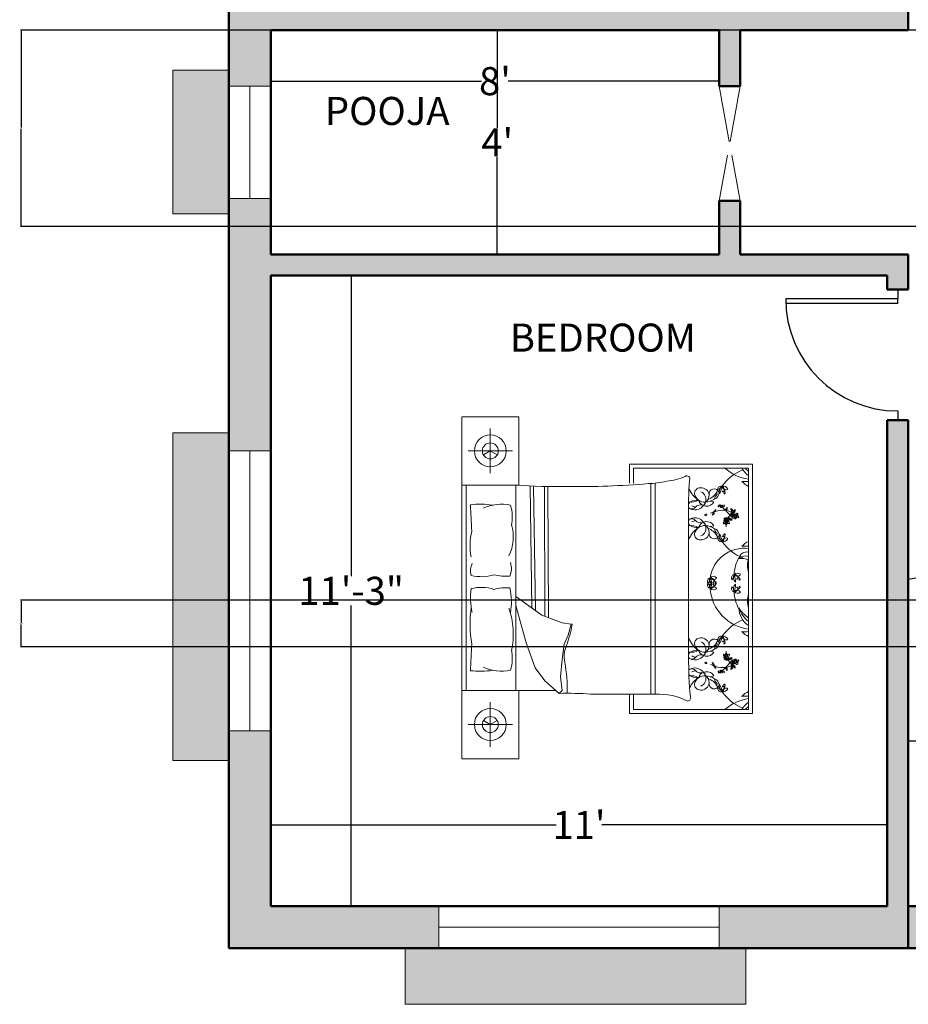
# Model space of a CAD drawing. Units: inches. Extents: x -28 to 544, y -640 to 52.
# Tile 1 of 11: x -28 to 162, y -600 to -389. Entities that reach past the tile are written whole.
import ezdxf

# ---------------------------------------------------------------- set-up
doc = ezdxf.new("R2010")
doc.units = ezdxf.units.IN
doc.header["$MEASUREMENT"] = 0
doc.linetypes.add('ACAD_ISO02W100', pattern=[15, 12, -3])
for name, color, linetype, lineweight in [('A-ANNO-DIMS', 2, 'Continuous', 18), ('A-AREA-IDEN', 7, 'Continuous', 25), ('A-DOOR', 3, 'Continuous', 25), ('A-FURN', 8, 'Continuous', 18), ('A-GLAZ', 4, 'Continuous', 20), ('A-ROOF', 8, 'Continuous', 18), ('A-ROOF-PATT', 252, 'Continuous', 13), ('A-WALL', 7, 'Continuous', 50), ('A-WALL-OVHD', 8, 'ACAD_ISO02W100', 18), ('A-WALL-PATT', 5, 'Continuous', 13)]:
    doc.layers.add(name, color=color, linetype=linetype, lineweight=lineweight)
doc.styles.get("Standard").update_dxf_attribs({"font": 'arial.ttf'})
doc.dimstyles.get("Standard").update_dxf_attribs({"dimtxt": 0.18, "dimasz": 0.18, "dimexe": 0.18, "dimexo": 0.0625, "dimgap": 0.09, "dimtad": 0, "dimtih": 1, "dimtoh": 1, "dimdec": 0, "dimzin": 0, "dimdsep": 46, "dimlunit": 3, "dimtxsty": 'Standard', "dimcen": 0.09, "dimadec": 0, "dimazin": 0, "dimtfac": 1, "dimtdec": 0, "dimtofl": 0, "dimtmove": 0, "dimatfit": 3, "dimfxl": 1, "dimtolj": 1, "dimtzin": 0, "dimarcsym": 0})

# ---------------------------------------------------------------- blocks, each defined once
blk = doc.blocks.new('*D21')
at = {"layer": 'A-ANNO-DIMS', "color": 0, "lineweight": -2, "transparency": 16777216}
for p, q in [((42.28, -443.74), (43.33, -443.74)), ((43.15, -443.92), (43.15, -508.09)), ((43.15, -578.56), (43.15, -514.4)), ((42.28, -578.74), (43.33, -578.74))]:
    blk.add_line(p, q, dxfattribs=at)
at = {"layer": 'A-ANNO-DIMS', "color": 0, "transparency": 16777216}
for points in [[(43.12, -443.92), (43.18, -443.92), (43.15, -443.74)], [(43.12, -578.56), (43.18, -578.56), (43.15, -578.74)]]:
    blk.add_solid(points, dxfattribs=at)
at = {"layer": 'Defpoints', "color": 0, "transparency": 16777216}
for p in [(42.22, -443.74), (42.22, -578.74), (43.15, -578.74)]:
    blk.add_point(p, dxfattribs=at)
at = {"layer": 'A-ANNO-DIMS', "color": 0, "transparency": 16777216, "insert": (43.15, -511.24), "char_height": 6, "attachment_point": 5}
blk.add_mtext('\\A1;11\'-3"', dxfattribs=at)
blk = doc.blocks.new('*D22')
at = {"layer": 'A-ANNO-DIMS', "color": 0, "lineweight": -2, "transparency": 16777216}
for p, q in [((25.94, -561.29), (25.94, -561.17)), ((26.12, -561.35), (87.05, -561.35)), ((157.76, -561.35), (96.84, -561.35)), ((157.94, -561.29), (157.94, -561.17))]:
    blk.add_line(p, q, dxfattribs=at)
at = {"layer": 'A-ANNO-DIMS', "color": 0, "transparency": 16777216}
for points in [[(26.12, -561.32), (26.12, -561.38), (25.94, -561.35)], [(157.76, -561.32), (157.76, -561.38), (157.94, -561.35)]]:
    blk.add_solid(points, dxfattribs=at)
at = {"layer": 'Defpoints', "color": 0, "transparency": 16777216}
for p in [(25.94, -561.35), (157.94, -561.35), (157.94, -561.35)]:
    blk.add_point(p, dxfattribs=at)
at = {"layer": 'A-ANNO-DIMS', "color": 0, "transparency": 16777216, "insert": (91.94, -561.35), "char_height": 6, "attachment_point": 5}
blk.add_mtext("\\A1;11'", dxfattribs=at)
blk = doc.blocks.new('*D29')
at = {"layer": 'A-ANNO-DIMS', "color": 0, "lineweight": -2, "transparency": 16777216}
for p, q in [((75.12, -391.24), (74.25, -391.24)), ((74.43, -391.42), (74.43, -412.15)), ((74.43, -439.06), (74.43, -418.33)), ((75.12, -439.24), (74.25, -439.24))]:
    blk.add_line(p, q, dxfattribs=at)
at = {"layer": 'A-ANNO-DIMS', "color": 0, "transparency": 16777216}
for points in [[(74.4, -391.42), (74.46, -391.42), (74.43, -391.24)], [(74.4, -439.06), (74.46, -439.06), (74.43, -439.24)]]:
    blk.add_solid(points, dxfattribs=at)
at = {"layer": 'Defpoints', "color": 0, "transparency": 16777216}
for p in [(75.19, -391.24), (74.43, -439.24), (75.19, -439.24)]:
    blk.add_point(p, dxfattribs=at)
at = {"layer": 'A-ANNO-DIMS', "color": 0, "transparency": 16777216, "insert": (74.43, -415.24), "char_height": 6, "attachment_point": 5}
blk.add_mtext("\\A1;4'", dxfattribs=at)
blk = doc.blocks.new('*D30')
at = {"layer": 'A-ANNO-DIMS', "color": 0, "lineweight": -2, "transparency": 16777216}
for p, q in [((25.94, -427.18), (25.94, -401.96)), ((26.12, -402.14), (71.09, -402.14)), ((121.76, -402.14), (76.8, -402.14)), ((121.94, -401.16), (121.94, -402.32))]:
    blk.add_line(p, q, dxfattribs=at)
at = {"layer": 'A-ANNO-DIMS', "color": 0, "transparency": 16777216}
for points in [[(26.12, -402.11), (26.12, -402.17), (25.94, -402.14)], [(121.76, -402.11), (121.76, -402.17), (121.94, -402.14)]]:
    blk.add_solid(points, dxfattribs=at)
at = {"layer": 'Defpoints', "color": 0, "transparency": 16777216}
for p in [(121.94, -401.09), (121.94, -402.14), (25.94, -427.24)]:
    blk.add_point(p, dxfattribs=at)
at = {"layer": 'A-ANNO-DIMS', "color": 0, "transparency": 16777216, "insert": (73.94, -402.14), "char_height": 6, "attachment_point": 5}
blk.add_mtext("\\A1;8'", dxfattribs=at)
blk = doc.blocks.new('*D41')
at = {"layer": 'A-ANNO-DIMS', "color": 0, "lineweight": -2, "transparency": 16777216}
for p, q in [((162.44, -543.27), (162.44, -543.15)), ((162.62, -543.33), (238.58, -543.33)), ((334.76, -543.33), (258.81, -543.33)), ((334.94, -543.27), (334.94, -543.15))]:
    blk.add_line(p, q, dxfattribs=at)
at = {"layer": 'A-ANNO-DIMS', "color": 0, "transparency": 16777216}
for points in [[(162.62, -543.3), (162.62, -543.36), (162.44, -543.33)], [(334.76, -543.3), (334.76, -543.36), (334.94, -543.33)]]:
    blk.add_solid(points, dxfattribs=at)
at = {"layer": 'Defpoints', "color": 0, "transparency": 16777216}
for p in [(162.44, -543.33), (334.94, -543.33), (334.94, -543.33)]:
    blk.add_point(p, dxfattribs=at)
at = {"layer": 'A-ANNO-DIMS', "color": 0, "transparency": 16777216, "insert": (248.69, -543.33), "char_height": 6, "attachment_point": 5}
blk.add_mtext('\\A1;14\'-5"', dxfattribs=at)
blk = doc.blocks.new('BED-DOUBLE-HEADBOARD-73')
for p, q in [((0, 0), (0, 73.21)), ((6.1, 61.11), (6.1, 70.67)), ((10.88, 65.89), (1.32, 65.89)), ((35.89, 58.98), (35.89, 63.04)), ((35.89, 63.04), (62.26, 63.04)), ((36.74, 62.19), (36.74, 58.96)), ((61.41, 62.19), (36.74, 62.19)), ((61.41, 10.51), (61.41, 62.19)), ((62.26, 63.04), (62.26, 9.66)), ((0.94, 58.57), (0.94, 14.64)), ((11.57, 14.64), (11.57, 58.57)), ((14.61, 58.37), (14.98, 32.31)), ((15.36, 58.34), (15.74, 31.76)), ((17.67, 58.31), (17.78, 30.51)), ((18.42, 58.31), (18.53, 30.22)), ((40.45, 58.9), (40.45, 13.8)), ((41.37, 58.97), (41.37, 13.8)), ((53.99, 54.97), (53.16, 55.14)), ((48.56, 51.47), (48.56, 21.74)), ((53.99, 49.86), (53.16, 49.7)), ((11.57, 34.76), (17.15, 30.74)), ((13.75, 24.81), (11.57, 32.8)), ((17.15, 30.74), (21.45, 29.11)), ((21.45, 29.11), (23.38, 28.82)), ((23.38, 28.82), (22.79, 26.44)), ((22.79, 26.44), (21.9, 24.52)), ((15.67, 19.47), (13.75, 24.81)), ((21.9, 24.52), (21.45, 21.25)), ((21.45, 21.25), (21.15, 17.55)), ((53.99, 22.84), (53.16, 23)), ((17.75, 16.66), (15.67, 19.47)), ((21.15, 17.55), (21.45, 14.58)), ((53.99, 17.73), (53.16, 17.56)), ((20.86, 13.99), (17.75, 16.66)), ((0, 14.64), (20.09, 14.64)), ((21.45, 14.58), (20.86, 13.99)), ((35.89, 9.66), (35.89, 13.8)), ((36.74, 13.8), (36.74, 10.51)), ((6.1, 12.1), (6.1, 2.54)), ((62.26, 9.66), (35.89, 9.66)), ((36.74, 10.51), (61.41, 10.51)), ((10.88, 7.32), (1.32, 7.32))]:
    blk.add_line(p, q)
for points in [[(0, 58.57), (12.2, 58.57), (12.2, 73.21), (0, 73.21)], [(6.1, 65.89), (4.62, 65.04)], [(6.1, 65.89), (7.58, 65.04)], [(12.2, 14.64), (12.2, 0), (0, 0)], [(6.1, 7.32), (4.62, 8.18)], [(6.1, 7.32), (7.58, 8.18)]]:
    blk.add_lwpolyline(points)
for points in [[(39.88, 58.88, 0.056112), (43.91, 59.41, 0.095341), (47.79, 60.44)], [(1.82, 54.36, -0.074897), (6.61, 54.28, 0.472817)], [(6.87, 39.39, -0.14099), (2, 39.24, -0.235245)], [(6.87, 36.26, 0.14099), (2, 36.41, 0.235245)], [(1.82, 18.85, 0.074897), (6.61, 18.94, -0.472817)], [(27.56, 13.83, 0.001242), (41.45, 13.8, -0.127202), (48.38, 12.33)]]:
    blk.add_lwpolyline(points, format="xyb")
for centre, radius in [((6.1, 65.89), 3.42), ((6.1, 65.89), 1.71), ((56.64, 50.74), 0.186), ((58.61, 51.96), 0.186), ((56.64, 21.96), 0.186), ((58.61, 20.74), 0.186), ((6.1, 7.32), 3.42), ((6.1, 7.32), 1.71)]:
    blk.add_circle(centre, radius)
for centre, radius, start, end in [((63.65, 52.95), 9.56, 111.4092, 145.6135), ((62.7, 69.31), 9.56, 228.1144, 262.255), ((63.98, 64.51), 4.66, 209.8884, 236.5383), ((64.85, 66.19), 5.81, 223.5186, 233.6964), ((48.16, 59.89), 0.667, 336.5219, 123.8264), ((119.76, 53.71), 71.24, 175.2402, 181.8035), ((62.9, 61.9), 3.89, 221.0454, 247.4453), ((60.81, 72.55), 13.23, 266.3481, 272.5919), ((20.52, 189.81), 131.55, 266.1, 270.9282), ((25.3, 229.86), 171.6, 269.1145, 274.8735), ((53.71, 59.98), 5.54, 203.6453, 236.3329), ((51.05, 56.75), 1.24, 88.9462, 185.5144), ((51.23, 56.25), 1.75, 7.1143, 95.0551), ((50.57, 55.56), 1.7, 338.5779, 68.4181), ((51.63, 58.83), 3.46, 288.2955, 328.7386), ((54.05, 56.65), 1.1, 19.1312, 189.736), ((53.72, 56.91), 1.37, 285.6955, 4.031), ((55.24, 56.88), 0.673, 126.7319, 206.0245), ((55.57, 57.58), 0.793, 76.272, 177.0484), ((54.36, 59.2), 1.63, 284.7031, 328.6173), ((56.64, 57.12), 1.51, 125.7657, 194.5347), ((49.23, 59.8), 6.69, 332.8176, 347.4827), ((55.98, 57.31), 1.06, 20.9613, 102.2885), ((56.55, 58.37), 0.798, 181.7131, 301.5367), ((53.94, 56.76), 2.42, 2.0648, 41.1598), ((55.39, 57.66), 0.782, 316.2238, 62.3173), ((55.84, 57.2), 0.0623, 20.2667, 316.2271), ((56.17, 56.85), 0.0577, 52.0591, 168.5166), ((49.1, 57.95), 3.03, 259.249, 301.1782), ((49.37, 54.19), 0.882, 127.675, 162.5814), ((49.89, 55.6), 2.33, 240.8249, 340.7178), ((50.42, 52.56), 2.82, 85.2696, 124.215), ((51.97, 57.13), 2.2, 193.079, 274.7067), ((52.41, 55.88), 1.82, 196.8663, 330.0915), ((51.65, 54.73), 0.454, 254.8529, 12.6959), ((50.42, 52.56), 2.82, 53.6555, 57.2989), ((50.84, 56.55), 2.13, 305.9599, 357.6409), ((51.91, 58.86), 3.93, 273.4924, 303.7117), ((55.54, 55.43), 1.46, 128.4175, 173.8338), ((56.23, 56.84), 0.119, 168.5166, 2.0648), ((-694.9, 14.01), 697.9, 2.85022, 3.31479), ((8.53, 45.04), 9.44, 78.2417, 114.8684), ((0.97, 51.75), 9.81, 348.9631, 14.8961), ((49.37, 54.19), 0.882, 196.6343, 225.5483), ((49.19, 54.56), 1.1, 246.1646, 318.4347), ((50.31, 55.95), 2.1, 240.0851, 262.564), ((51.14, 52.84), 1.5, 74.8529, 138.4347), ((56.02, 47.13), 6.06, 110.1059, 116.9968), ((53.95, 52.6), 0.149, 83.9457, 185.6216), ((53.35, 52.74), 0.614, 328.836, 0.8141), ((53.67, 52.56), 0.351, 306.5232, 32.4668), ((54.09, 52.83), 0.149, 112.5583, 214.2343), ((53.99, 53.1), 0.351, 265.7131, 351.6568), ((53.68, 53.29), 0.614, 297.3659, 329.344), ((53.22, 53.82), 1.18, 313.6929, 321.7899), ((54.52, 53.01), 0.384, 115.5379, 168.6744), ((53.21, 53.57), 1.16, 329.344, 349.7412), ((56.02, 47.13), 6.06, 86.1723, 106.4158), ((52.29, 53.3), 2.06, 352.8698, 1.6736), ((55.02, 54.05), 0.144, 125.0752, 284.7644), ((55.25, 54.1), 0.311, 127.3642, 168.4363), ((55, 54.35), 0.448, 277.4968, 341.2737), ((55.36, 54.14), 0.178, 88.1325, 178.8919), ((55.72, 53.95), 0.385, 136.3462, 189.6513), ((55.5, 53.92), 0.161, 189.6513, 312.3208), ((55.54, 54.36), 0.186, 183.2768, 356.7232), ((56.12, 54.03), 0.61, 164.2829, 186.9148), ((55.4, 54.02), 0.305, 312.3208, 40.2111), ((56.04, 54.37), 0.433, 201.6382, 274.947), ((55.47, 53.77), 0.566, 42.3896, 66.5724), ((61.18, 58.25), 6.95, 217.9541, 226.8459), ((55.88, 54.11), 0.308, 10.9597, 52.2379), ((56.07, 54.08), 0.143, 274.947, 37.5263), ((56.55, 53.27), 0.149, 112.5583, 214.2343), ((56.45, 53.53), 0.351, 265.7131, 351.6568), ((56.14, 53.73), 0.614, 297.3659, 329.344), ((56.17, 50.15), 3.04, 60.7959, 85.244), ((49.7, 45.78), 10, 37.8256, 47.7588), ((55.68, 54.25), 1.18, 313.6929, 321.7899), ((56.98, 53.45), 0.384, 115.5379, 168.6744), ((55.68, 54), 1.16, 329.344, 349.7412), ((54.75, 53.74), 2.06, 352.8698, 1.6736), ((57.66, 53.32), 0.208, 33.0979, 123.1364), ((53.07, 50.39), 5.45, 31.1156, 34.8118), ((57.35, 52.96), 0.564, 2.3172, 70.5201), ((57.82, 52.83), 0.163, 135.7354, 318.1297), ((57.55, 53.09), 0.216, 315.7354, 31.1156), ((57.94, 52.83), 0.163, 68.2452, 250.6395), ((57.57, 53.03), 0.485, 352.6008, 57.1845), ((59.3, 49.77), 3.25, 111.7087, 116.2181), ((58.03, 53.14), 0.485, 252.8042, 349.6943), ((58.08, 53.18), 0.216, 248.2452, 323.6254), ((57.89, 53.31), 0.564, 291.7087, 3.0299), ((53.87, 56.28), 5.45, 323.6254, 327.3216), ((58.34, 53.17), 0.208, 325.6077, 55.6462), ((49.37, 50.64), 0.882, 134.4517, 156.7144), ((49.89, 49.23), 2.33, 19.2822, 119.1751), ((49.19, 50.27), 1.1, 41.5653, 113.8354), ((50.31, 48.88), 2.1, 97.436, 119.9149), ((51.14, 51.99), 1.5, 221.5653, 285.1471), ((52.41, 48.95), 1.82, 29.9085, 163.1337), ((52.25, 52.22), 0.229, 169.5864, 349.5616), ((52.34, 52.21), 0.141, 349.5616, 167.2949), ((53.99, 52.13), 0.384, 129.5056, 182.6421), ((52.88, 53.02), 1.16, 308.4388, 328.836), ((52.68, 53.96), 2.06, 296.5064, 305.3102), ((52.67, 52.9), 1.18, 336.3901, 344.4871), ((56.35, 50.49), 0.311, 93.635, 168.4363), ((56.37, 52.17), 0.85, 253.6301, 325.4631), ((56.6, 50.99), 0.601, 82.0748, 142.6895), ((56.54, 51.82), 0.617, 228.342, 274.9894), ((56.31, 50.98), 0.183, 138.2946, 276.2474), ((56.11, 50.74), 0.448, 277.4968, 341.2737), ((56.38, 50.95), 0.254, 358.5719, 143.8954), ((56.47, 50.53), 0.178, 88.1325, 178.8919), ((56.53, 51.15), 0.257, 208.8493, 269.9355), ((56.31, 51.09), 0.293, 274.2123, 318.1587), ((56.83, 50.34), 0.385, 136.3462, 189.6513), ((56.56, 51.72), 0.517, 273.8774, 357.1501), ((57.21, 50.79), 0.588, 121.9501, 165.2442), ((56.76, 52.08), 0.5, 262.0748, 308.2393), ((56.51, 50.41), 0.305, 312.3208, 40.2111), ((57.15, 50.75), 0.433, 201.6382, 274.947), ((56.8, 51.02), 0.123, 262.868, 7.094), ((56.58, 50.16), 0.566, 42.3896, 66.5724), ((56.79, 51.12), 0.368, 278.5614, 22.5914), ((56.99, 50.49), 0.308, 10.9597, 118.7804), ((60.21, 49.84), 3.65, 156.1523, 156.9499), ((56.99, 51.14), 0.185, 44.3732, 121.9501), ((57.56, 51.57), 0.517, 181.4625, 249.4747), ((60.21, 49.84), 3.65, 130.182, 149.456), ((57.48, 51.98), 0.5, 215.1128, 261.2773), ((57.88, 51.95), 0.85, 197.889, 269.722), ((57.61, 51.66), 0.617, 248.3627, 295.0101), ((57.31, 50.89), 0.601, 20.6625, 81.2773), ((58.2, 51.92), 0.601, 139.3812, 199.9959), ((57.08, 52.35), 0.85, 310.9365, 22.7695), ((57.47, 52.31), 0.617, 285.6484, 332.2957), ((57.37, 52.63), 0.5, 319.3812, 5.5456), ((56.17, 50.15), 3.04, 47.5083, 55.9967), ((57.57, 52.27), 0.517, 331.1838, 51.6792), ((58.1, 51.65), 0.144, 125.0752, 284.7644), ((58.32, 51.71), 0.311, 93.635, 168.4363), ((58.28, 52.2), 0.183, 138.2946, 276.2474), ((58.08, 51.96), 0.448, 277.4968, 341.2737), ((58.35, 52.17), 0.254, 358.5719, 143.8954), ((58.43, 51.75), 0.178, 88.1325, 178.8919), ((58.5, 52.37), 0.257, 208.8493, 269.9355), ((58.28, 52.31), 0.293, 274.2123, 318.1587), ((58.79, 51.56), 0.385, 136.3462, 189.6513), ((58.57, 51.52), 0.161, 189.6513, 312.3208), ((59.19, 51.63), 0.61, 164.2829, 186.9148), ((59.17, 52.01), 0.588, 121.9501, 165.2442), ((58.47, 51.63), 0.305, 312.3208, 40.2111), ((59.12, 51.97), 0.433, 201.6382, 274.947), ((58.77, 52.24), 0.123, 262.868, 7.094), ((58.54, 51.38), 0.566, 42.3896, 66.5724), ((58.75, 52.34), 0.368, 278.5614, 22.5914), ((58.95, 51.71), 0.308, 10.9597, 118.7804), ((58.96, 52.36), 0.185, 44.3732, 121.9501), ((59.14, 51.68), 0.143, 274.947, 37.5263), ((14.63, 45.68), 12.87, 166.3427, 191.1841), ((1.69, 47.52), 9.32, 333.8761, 16.1746), ((49.37, 50.64), 0.882, 203.2856, 232.325), ((49.1, 46.88), 3.03, 58.8218, 100.2867), ((53.71, 44.85), 5.54, 123.6671, 158.5059), ((50.42, 52.28), 2.82, 235.785, 274.7304), ((51.97, 47.7), 2.2, 85.2933, 166.921), ((50.57, 49.27), 1.7, 291.5819, 21.4221), ((51.65, 50.1), 0.454, 347.3041, 105.1471), ((50.42, 52.28), 2.82, 302.7011, 306.3445), ((50.84, 48.28), 2.13, 2.3591, 54.0401), ((51.91, 45.97), 3.93, 56.2883, 86.5076), ((51.63, 46), 3.46, 31.2614, 71.7045), ((55.54, 49.4), 1.46, 186.1662, 231.5825), ((53.72, 47.92), 1.37, 355.969, 74.3045), ((56.13, 50.43), 0.144, 125.0752, 284.7644), ((56.6, 50.3), 0.161, 189.6513, 312.3208), ((60.21, 49.84), 3.65, 175.2415, 182.8929), ((57.23, 50.41), 0.61, 164.2829, 186.9148), ((57.18, 50.46), 0.143, 274.947, 37.5263), ((51.05, 48.08), 1.24, 174.4856, 271.0538), ((51.23, 48.59), 1.75, 264.9449, 352.8857), ((54.05, 48.18), 1.1, 170.264, 340.8688), ((55.24, 47.96), 0.673, 153.9755, 233.2681), ((55.57, 47.25), 0.793, 182.9516, 283.728), ((54.36, 45.63), 1.63, 31.3827, 75.2969), ((56.64, 47.71), 1.51, 165.4653, 234.2343), ((49.23, 45.03), 6.69, 12.5173, 27.1824), ((53.94, 48.07), 2.42, 318.8402, 357.9352), ((55.39, 47.18), 0.782, 297.6827, 43.7762), ((56.55, 46.46), 0.798, 58.4633, 178.2869), ((55.98, 47.52), 1.06, 257.7115, 339.0387), ((63.65, 51.88), 9.56, 214.3865, 248.5908), ((55.88, 47.64), 0.103, 43.7762, 339.7183), ((56.23, 47.99), 0.119, 357.9352, 191.4834), ((56.17, 47.98), 0.0577, 191.4834, 307.9409), ((62.9, 42.93), 3.89, 112.5547, 138.9546), ((60.49, 37.66), 7.4, 82.8636, 171.8197), ((60.81, 32.28), 13.23, 87.4081, 93.6519), ((67.82, 38.7), 9.56, 152.5854, 175.5377), ((61.01, 42.54), 1.72, 76.3898, 169.0739), ((60.77, 41.25), 2.17, 72.8609, 131.9049), ((59.82, 38.61), 4.28, 68.117, 96.6195), ((66.44, 41.37), 5.26, 162.9798, 196.4569), ((5.48, 40.25), 3.62, 153.3437, 196.1026), ((6.74, 40.74), 3.88, 335.0183, 18.5407), ((69.15, 39.29), 7.77, 174.3643, 175.6213), ((9.32, 48.02), 8.97, 254.1707, 275.9871), ((53.39, 37.95), 0.793, 106.1963, 206.9726), ((51.54, 38.75), 1.63, 314.6273, 358.5415), ((54.55, 38.09), 1.51, 155.6899, 224.4589), ((54.55, 37.05), 1.51, 135.5411, 204.3101), ((53.88, 37.92), 1.06, 50.8855, 132.2127), ((53.85, 39.13), 0.798, 211.6373, 331.4609), ((53.2, 37.93), 0.782, 346.148, 92.2415), ((52.39, 36.42), 2.42, 31.989, 71.0841), ((46.79, 36.71), 6.69, 2.7418, 17.407), ((46.79, 38.43), 6.69, 342.593, 357.2582), ((58.51, 38.68), 0.793, 106.1963, 206.9726), ((56.66, 39.48), 1.63, 314.6273, 358.5415), ((59.67, 38.82), 1.51, 155.6899, 224.4589), ((59, 38.66), 1.06, 50.8855, 132.2127), ((58.97, 39.86), 0.798, 211.6373, 331.4609), ((57.51, 37.15), 2.42, 31.989, 71.0841), ((51.91, 37.44), 6.69, 2.7418, 17.407), ((58.32, 38.66), 0.782, 346.148, 92.2415), ((58.94, 38.49), 0.0623, 50.1909, 346.0209), ((59.46, 38.37), 0.119, 198.4408, 31.989), ((59.4, 38.35), 0.0577, 81.9833, 198.4408), ((74.47, 35.19), 13.89, 160.0972, 160.2783), ((14.9, 34.49), 13.05, 171.5249, 193.96), ((9.32, 27.63), 8.97, 84.0129, 105.8293), ((-2.29, 33.51), 12.91, 349.8617, 13.6238), ((53.39, 37.19), 0.793, 153.0274, 253.8037), ((51.54, 36.39), 1.63, 1.4585, 45.3727), ((52.39, 38.72), 2.42, 288.9159, 328.011), ((53.2, 37.21), 0.782, 267.7585, 13.852), ((53.85, 36.01), 0.798, 28.5391, 148.3627), ((53.88, 37.22), 1.06, 227.7873, 309.1145), ((62.7, 37.18), 9.56, 184.4623, 262.255), ((53.82, 37.76), 0.0623, 50.1909, 346.0209), ((53.86, 37.38), 0.103, 13.852, 309.9245), ((54.34, 37.64), 0.119, 198.4408, 31.989), ((54.28, 37.62), 0.0577, 81.9833, 198.4408), ((54.34, 37.5), 0.119, 328.011, 161.5592), ((54.28, 37.52), 0.0577, 161.5592, 278.0167), ((58.51, 36.46), 0.793, 153.0274, 253.8037), ((56.66, 35.66), 1.63, 1.4585, 45.3727), ((59.67, 36.32), 1.51, 135.5411, 204.3101), ((51.91, 37.7), 6.69, 342.593, 357.2582), ((57.51, 37.99), 2.42, 288.9159, 328.011), ((58.32, 36.48), 0.782, 267.7585, 13.852), ((58.97, 35.28), 0.798, 28.5391, 148.3627), ((58.98, 36.64), 0.103, 13.852, 309.9245), ((59.46, 36.77), 0.119, 328.011, 161.5592), ((59.4, 36.79), 0.0577, 161.5592, 278.0167), ((59, 36.48), 1.06, 227.7873, 309.1145), ((67.82, 36.44), 9.56, 184.4623, 207.4146), ((66.44, 33.77), 5.26, 163.5431, 197.0202), ((69.15, 35.85), 7.77, 184.3787, 185.6357), ((74.47, 39.95), 13.89, 199.7217, 199.9028), ((28.32, 28.88), 26.55, 172.2196, 189.497), ((-6.01, 26.62), 17.02, 348.0397, 19.2615), ((63.98, 32.38), 4.66, 181.272, 236.5383), ((66.48, 37.11), 8.64, 214.0123, 234.053), ((64.85, 34.06), 5.81, 197.8504, 233.6964), ((63.65, 20.82), 9.56, 111.4092, 145.6135), ((-4.29, 33.9), 28.39, 340.1194, 349.3383), ((23.44, 28.65), 0.177, 358.8623, 109.7536), ((53.71, 27.85), 5.54, 201.4941, 236.3329), ((51.05, 24.62), 1.24, 88.9462, 185.5144), ((51.23, 24.12), 1.75, 7.1143, 95.0551), ((54.05, 24.52), 1.1, 19.1312, 189.736), ((55.57, 25.45), 0.793, 76.272, 177.0484), ((54.36, 27.07), 1.63, 284.7031, 328.6173), ((56.64, 24.99), 1.51, 125.7657, 194.5347), ((49.23, 27.67), 6.69, 332.8176, 347.4827), ((55.98, 25.18), 1.06, 20.9613, 102.2885), ((55.39, 25.53), 0.782, 316.2238, 62.3173), ((53.94, 24.63), 2.42, 2.0648, 41.1598), ((56.55, 26.24), 0.798, 181.7131, 301.5367), ((60.81, 40.42), 13.23, 266.3481, 272.5919), ((62.9, 29.77), 3.89, 221.0454, 247.4453), ((-694.9, 59.2), 697.9, 356.68521, 357.14978), ((0.97, 21.46), 9.81, 345.1039, 11.0369), ((27.87, 21.84), 5.96, 156.2616, 191.3392), ((49.1, 25.82), 3.03, 259.7133, 301.1782), ((50.42, 20.42), 2.82, 85.2696, 124.215), ((51.97, 25), 2.2, 193.079, 274.7067), ((52.41, 23.75), 1.82, 196.8663, 330.0915), ((50.57, 23.43), 1.7, 338.5779, 68.4181), ((50.84, 24.42), 2.13, 305.9599, 357.6409), ((51.91, 26.73), 3.93, 273.4924, 303.7117), ((51.63, 26.7), 3.46, 288.2955, 328.7386), ((53.72, 24.78), 1.37, 285.6955, 4.031), ((55.54, 23.3), 1.46, 128.4175, 173.8338), ((55.24, 24.74), 0.673, 126.7319, 206.0245), ((55.84, 25.07), 0.0623, 20.2667, 316.2271), ((56.17, 24.72), 0.0577, 52.0591, 168.5166), ((56.23, 24.71), 0.119, 168.5166, 2.0648), ((124.77, 20.87), 76.21, 179.3433, 185.6887), ((49.37, 22.06), 0.882, 127.675, 156.7144), ((49.37, 22.06), 0.882, 203.229, 225.5483), ((49.89, 23.47), 2.33, 240.8249, 340.7178), ((49.19, 22.43), 1.1, 246.1646, 318.4347), ((50.31, 23.82), 2.1, 240.0851, 262.564), ((51.14, 20.71), 1.5, 74.8529, 138.4347), ((51.65, 22.6), 0.454, 254.8529, 12.6959), ((50.42, 20.42), 2.82, 53.6555, 57.2989), ((56.13, 22.27), 0.144, 75.2356, 234.9248), ((56.35, 22.21), 0.311, 191.5637, 266.365), ((56.31, 21.72), 0.183, 83.7526, 221.7054), ((56.54, 20.88), 0.617, 85.0106, 131.658), ((56.37, 20.53), 0.85, 34.5369, 106.3699), ((56.6, 21.71), 0.601, 217.3105, 277.9252), ((56.11, 21.96), 0.448, 18.7263, 82.5032), ((56.38, 21.75), 0.254, 216.1046, 1.4281), ((56.47, 22.17), 0.178, 181.1081, 271.8675), ((56.53, 21.55), 0.257, 90.0645, 151.1507), ((56.31, 21.61), 0.293, 41.8413, 85.7877), ((56.83, 22.36), 0.385, 170.3487, 223.6538), ((56.6, 22.4), 0.161, 47.6792, 170.3487), ((60.21, 22.86), 3.65, 177.1071, 184.7585), ((56.56, 20.98), 0.517, 2.8499, 86.1226), ((57.23, 22.29), 0.61, 173.0852, 195.7171), ((57.21, 21.91), 0.588, 194.7558, 238.0499), ((56.76, 20.62), 0.5, 51.7607, 97.9252), ((56.51, 22.29), 0.305, 319.7889, 47.6792), ((57.15, 21.95), 0.433, 85.053, 158.3618), ((56.8, 21.68), 0.123, 352.906, 97.132), ((56.58, 22.54), 0.566, 293.4276, 317.6104), ((56.99, 22.21), 0.308, 241.2196, 349.0403), ((56.79, 21.58), 0.368, 337.4086, 81.4386), ((60.21, 22.86), 3.65, 203.0501, 203.8477), ((56.99, 21.56), 0.185, 238.0499, 315.6268), ((57.56, 21.13), 0.517, 110.5253, 178.5375), ((57.88, 20.75), 0.85, 90.278, 162.111), ((57.48, 20.72), 0.5, 98.7227, 144.8872), ((57.18, 22.24), 0.143, 322.4737, 85.053), ((57.61, 21.04), 0.617, 64.9899, 111.6373), ((57.31, 21.81), 0.601, 278.7227, 339.3375), ((58.1, 21.05), 0.144, 75.2356, 234.9248), ((58.08, 20.74), 0.448, 18.7263, 82.5032), ((58.79, 21.14), 0.385, 170.3487, 223.6538), ((58.57, 21.18), 0.161, 47.6792, 170.3487), ((59.19, 21.07), 0.61, 173.0852, 195.7171), ((58.47, 21.07), 0.305, 319.7889, 47.6792), ((59.12, 20.73), 0.433, 85.053, 158.3618), ((59.14, 21.02), 0.143, 322.4737, 85.053), ((8.53, 28.17), 9.44, 245.1316, 281.7583), ((-5.07, 15.24), 27.63, 357.4519, 11.3392), ((49.37, 18.51), 0.882, 134.4517, 153.558), ((49.89, 17.1), 2.33, 19.2822, 119.1751), ((49.19, 18.14), 1.1, 41.5653, 113.8354), ((52.25, 20.48), 0.229, 10.4384, 190.4136), ((52.34, 20.49), 0.141, 192.7051, 10.4384), ((56.02, 25.57), 6.06, 243.0032, 249.8941), ((52.88, 19.68), 1.16, 31.164, 51.5612), ((53.99, 20.57), 0.384, 177.3579, 230.4944), ((52.68, 18.74), 2.06, 54.6898, 63.4936), ((52.67, 19.8), 1.18, 15.5129, 23.6099), ((53.95, 20.1), 0.149, 174.3784, 276.0543), ((53.35, 19.96), 0.614, 359.1859, 31.164), ((53.67, 20.14), 0.351, 327.5332, 53.4768), ((54.09, 19.87), 0.149, 145.7657, 247.4417), ((53.99, 19.61), 0.351, 8.3432, 94.2869), ((53.68, 19.41), 0.614, 30.656, 62.6341), ((53.22, 18.88), 1.18, 38.2101, 46.3071), ((54.52, 19.69), 0.384, 191.3256, 244.4621), ((53.21, 19.13), 1.16, 10.2588, 30.656), ((56.02, 25.57), 6.06, 253.5842, 273.8277), ((52.29, 19.4), 2.06, 358.3264, 7.1302), ((61.18, 14.45), 6.95, 133.1541, 142.0459), ((56.55, 19.44), 0.149, 145.7657, 247.4417), ((49.7, 26.92), 10, 312.2412, 322.1744), ((56.17, 22.55), 3.04, 274.756, 299.2041), ((56.45, 19.17), 0.351, 8.3432, 94.2869), ((56.14, 18.97), 0.614, 30.656, 62.6341), ((55.68, 18.45), 1.18, 38.2101, 46.3071), ((56.98, 19.25), 0.384, 191.3256, 244.4621), ((55.68, 18.7), 1.16, 10.2588, 30.656), ((54.75, 18.96), 2.06, 358.3264, 7.1302), ((60.21, 22.86), 3.65, 210.544, 229.818), ((57.35, 19.74), 0.564, 289.4799, 357.6828), ((53.07, 22.32), 5.45, 325.1882, 328.8844), ((57.66, 19.38), 0.208, 236.8636, 326.9021), ((58.2, 20.78), 0.601, 160.0041, 220.6188), ((57.08, 20.35), 0.85, 337.2305, 49.0635), ((57.47, 20.4), 0.617, 27.7043, 74.3516), ((57.82, 19.88), 0.163, 41.8703, 224.2646), ((57.55, 19.61), 0.216, 328.8844, 44.2646), ((57.37, 20.07), 0.5, 354.4544, 40.6188), ((57.94, 19.87), 0.163, 109.3605, 291.7548), ((57.57, 19.67), 0.485, 302.8155, 7.3992), ((56.17, 22.55), 3.04, 304.0033, 312.4917), ((59.3, 22.93), 3.25, 243.7819, 248.2913), ((57.57, 20.43), 0.517, 308.3208, 28.8162), ((58.03, 19.56), 0.485, 10.3057, 107.1958), ((58.08, 19.52), 0.216, 36.3746, 111.7548), ((58.32, 20.99), 0.311, 191.5637, 266.365), ((58.28, 20.5), 0.183, 83.7526, 221.7054), ((57.89, 19.39), 0.564, 356.9701, 68.2913), ((58.35, 20.53), 0.254, 216.1046, 1.4281), ((58.43, 20.95), 0.178, 181.1081, 271.8675), ((53.87, 16.42), 5.45, 32.6784, 36.3746), ((58.5, 20.33), 0.257, 90.0645, 151.1507), ((58.28, 20.39), 0.293, 41.8413, 85.7877), ((58.34, 19.53), 0.208, 304.3538, 34.3923), ((59.17, 20.69), 0.588, 194.7558, 238.0499), ((58.77, 20.46), 0.123, 352.906, 97.132), ((58.54, 21.32), 0.566, 293.4276, 317.6104), ((58.95, 20.99), 0.308, 241.2196, 349.0403), ((58.75, 20.36), 0.368, 337.4086, 81.4386), ((58.96, 20.34), 0.185, 238.0499, 315.6268), ((49.37, 18.51), 0.882, 210.0293, 232.325), ((49.1, 14.75), 3.03, 58.8218, 99.1554), ((53.71, 12.72), 5.54, 123.6671, 153.2997), ((50.42, 20.15), 2.82, 235.785, 274.7304), ((50.31, 16.75), 2.1, 97.436, 119.9149), ((51.97, 15.57), 2.2, 85.2933, 166.921), ((51.14, 19.86), 1.5, 221.5653, 285.1471), ((52.41, 16.82), 1.82, 29.9085, 163.1337), ((50.57, 17.14), 1.7, 291.5819, 21.4221), ((51.65, 17.97), 0.454, 347.3041, 105.1471), ((50.42, 20.15), 2.82, 302.7011, 306.3445), ((50.84, 16.15), 2.13, 2.3591, 54.0401), ((51.91, 13.84), 3.93, 56.2883, 86.5076), ((51.63, 13.87), 3.46, 31.2614, 71.7045), ((53.72, 15.79), 1.37, 355.969, 74.3045), ((55.54, 17.27), 1.46, 186.1662, 231.5825), ((55.02, 18.65), 0.144, 75.2356, 234.9248), ((55.25, 18.6), 0.311, 191.5637, 232.6358), ((55, 18.35), 0.448, 18.7263, 82.5032), ((55.36, 18.56), 0.178, 181.1081, 271.8675), ((55.72, 18.75), 0.385, 170.3487, 223.6538), ((55.5, 18.79), 0.161, 47.6792, 170.3487), ((55.54, 18.34), 0.186, 3.2768, 176.7232), ((56.12, 18.67), 0.61, 173.0852, 195.7171), ((55.4, 18.68), 0.305, 319.7889, 47.6792), ((56.04, 18.34), 0.433, 85.053, 158.3618), ((55.47, 18.93), 0.566, 293.4276, 317.6104), ((55.88, 18.6), 0.308, 307.7621, 349.0403), ((56.07, 18.62), 0.143, 322.4737, 85.053), ((51.05, 15.95), 1.24, 174.4856, 271.0538), ((51.23, 16.45), 1.75, 264.9449, 352.8857), ((54.05, 16.05), 1.1, 170.264, 340.8688), ((55.24, 15.83), 0.673, 153.9755, 233.2681), ((54.36, 13.5), 1.63, 31.3827, 75.2969), ((55.57, 15.12), 0.793, 182.9516, 283.728), ((56.64, 15.58), 1.51, 165.4653, 234.2343), ((49.23, 12.9), 6.69, 12.5173, 27.1824), ((53.94, 15.94), 2.42, 318.8402, 357.9352), ((55.39, 15.04), 0.782, 297.6827, 43.7762), ((56.55, 14.33), 0.798, 58.4633, 178.2869), ((55.98, 15.39), 1.06, 257.7115, 339.0387), ((55.88, 15.51), 0.103, 43.7762, 339.7183), ((56.23, 15.86), 0.119, 357.9352, 191.4834), ((56.17, 15.85), 0.0577, 191.4834, 307.9409), ((22.68, -53.14), 67.15, 85.8294, 91.553), ((48.33, 13.01), 0.676, 273.98, 27.3412), ((63.65, 19.75), 9.56, 214.3865, 248.5908), ((62.7, 3.39), 9.56, 97.745, 131.8856), ((62.9, 10.8), 3.89, 112.5547, 138.9546), ((60.81, 0.15), 13.23, 87.4081, 93.6519), ((63.98, 8.19), 4.66, 123.4617, 150.1116), ((64.85, 6.51), 5.81, 126.3036, 136.4814)]:
    blk.add_arc(centre, radius, start, end)
blk = doc.blocks.new('WIN-60IN')
for p, q in [((0, 9), (60, 9)), ((0, 0), (0, 9)), ((60, 9), (60, 0)), ((0, 4.5), (60, 4.5)), ((60, 0), (0, 0))]:
    blk.add_line(p, q)
blk = doc.blocks.new('WIN-24IN')
for p, q in [((0, 0), (0, 24)), ((0, 24), (9, 24)), ((4.5, 0), (4.5, 24)), ((9, 24), (9, 0)), ((9, 0), (0, 0))]:
    blk.add_line(p, q)
blk = doc.blocks.new('DOOR-SWING-24IN')
for p, q in [((25, 0), (25, 24)), ((26, 0), (26, 24)), ((2, 0), (0, 0)), ((25, 0), (26, 0)), ((28, 0), (26, 0))]:
    blk.add_line(p, q)
blk.add_arc((26, 0), 24, 90, 180)
blk = doc.blocks.new('*D82')
at = {"layer": 'A-ANNO-DIMS', "color": 0, "lineweight": -2, "transparency": 16777216}
for p, q in [((205.38, -513.24), (-27.66, -513.24)), ((-27.48, -513.42), (-27.48, -518.06)), ((-27.48, -523.06), (-27.48, -518.42)), ((205.38, -523.24), (-27.66, -523.24))]:
    blk.add_line(p, q, dxfattribs=at)
at = {"layer": 'A-ANNO-DIMS', "color": 0, "transparency": 16777216}
for points in [[(-27.51, -513.42), (-27.45, -513.42), (-27.48, -513.24)], [(-27.51, -523.06), (-27.45, -523.06), (-27.48, -523.24)]]:
    blk.add_solid(points, dxfattribs=at)
at = {"layer": 'Defpoints', "color": 0, "transparency": 16777216}
for p in [(-27.48, -513.24), (205.44, -513.24), (205.44, -523.24)]:
    blk.add_point(p, dxfattribs=at)
at = {"layer": 'A-ANNO-DIMS', "color": 0, "transparency": 16777216, "insert": (-27.48, -518.24), "char_height": 0.18, "attachment_point": 5}
blk.add_mtext('\\A1;0\'-10"', dxfattribs=at)
blk = doc.blocks.new('*D83')
at = {"layer": 'A-ANNO-DIMS', "color": 0, "lineweight": -2, "transparency": 16777216}
for p, q in [((205.38, -391.24), (-27.66, -391.24)), ((-27.48, -391.42), (-27.48, -412.06)), ((-27.48, -433.06), (-27.48, -412.42)), ((205.38, -433.24), (-27.66, -433.24))]:
    blk.add_line(p, q, dxfattribs=at)
at = {"layer": 'A-ANNO-DIMS', "color": 0, "transparency": 16777216}
for points in [[(-27.51, -391.42), (-27.45, -391.42), (-27.48, -391.24)], [(-27.51, -433.06), (-27.45, -433.06), (-27.48, -433.24)]]:
    blk.add_solid(points, dxfattribs=at)
at = {"layer": 'Defpoints', "color": 0, "transparency": 16777216}
for p in [(205.44, -391.24), (-27.48, -433.24), (205.44, -433.24)]:
    blk.add_point(p, dxfattribs=at)
at = {"layer": 'A-ANNO-DIMS', "color": 0, "transparency": 16777216, "insert": (-27.48, -412.24), "char_height": 0.18, "attachment_point": 5}
blk.add_mtext('\\A1;3\'-6"', dxfattribs=at)

msp = doc.modelspace()

# ---------------------------------------------------------------- hatches: boundary and pattern name
at = {"layer": 'A-ROOF-PATT'}
h = msp.add_hatch(color=256, dxfattribs=at)
h.dxf.hatch_style = 1
h.set_gradient(color1=(241, 235, 31), color2=(248, 153, 30))
h.paths.add_polyline_path([(124.53, 19.76), (58.75, 19.76), (58.75, 7.76), (124.53, 7.76)])
h.paths.add_polyline_path([(226.33, 19.76), (182.83, 19.76), (182.83, 7.76), (226.33, 7.76)])
h.paths.add_polyline_path([(313.67, 19.76), (271.84, 19.76), (271.84, 7.76), (313.67, 7.76)])
h.paths.add_polyline_path([(440.55, 19.76), (372.16, 19.76), (372.16, 7.76), (440.55, 7.76)])
h.paths.add_polyline_path([(492.44, -34.91), (480.44, -34.91), (480.44, -100.18), (492.44, -100.18)])
h.paths.add_polyline_path([(492.44, -151.37), (480.44, -151.37), (480.44, -179.02), (492.44, -179.02)])
h.paths.add_polyline_path([(492.44, -207.96), (480.44, -207.96), (480.44, -238.77), (492.44, -238.77)])
h.paths.add_polyline_path([(492.44, -289.99), (480.44, -289.99), (480.44, -354.53), (492.44, -354.53)])
h.paths.add_polyline_path([(492.44, -399.27), (480.44, -399.27), (480.44, -430), (492.44, -430)])
h.paths.add_polyline_path([(492.44, -475.99), (480.44, -475.99), (480.44, -546.14), (492.44, -546.14)])
h.paths.add_polyline_path([(442.7, -587.74), (368.43, -587.74), (368.43, -599.74), (442.7, -599.74)])
h.paths.add_polyline_path([(127.64, -587.74), (54.75, -587.74), (54.75, -599.74), (127.64, -599.74)])
h.paths.add_polyline_path([(16.94, -477.43), (4.94, -477.43), (4.94, -547.54), (16.94, -547.54)])
h.paths.add_polyline_path([(16.94, -399.8), (4.94, -399.8), (4.94, -430.58), (16.94, -430.58)])
h.paths.add_polyline_path([(16.94, -287.93), (4.94, -287.93), (4.94, -356.82), (16.94, -356.82)])
h.paths.add_polyline_path([(16.94, -208.93), (4.94, -208.93), (4.94, -240.18), (16.94, -240.18)])
h.paths.add_polyline_path([(16.94, -150), (4.94, -150), (4.94, -180.17), (16.94, -180.17)])
h.paths.add_polyline_path([(16.94, -32.89), (4.94, -32.89), (4.94, -101.73), (16.94, -101.73)])
at = {"layer": 'A-WALL-PATT'}
h = msp.add_hatch(color=256, dxfattribs=at)
h.dxf.hatch_style = 1
h.paths.add_polyline_path([(25.94, -235.24), (16.94, -235.24), (16.94, -290.74), (25.94, -290.74), (25.94, -254.74), (127.94, -254.74), (127.94, -252.49), (127.94, -250.24), (118.94, -250.24), (118.94, -247.24), (109.94, -247.24), (109.94, -250.24), (25.94, -250.24)])
h.paths.add_polyline_path([(114.44, -191.74), (114.44, -137.74), (126.94, -137.74), (126.94, -135.49), (126.94, -133.24), (109.94, -133.24), (109.94, -137.74), (109.94, -191.74), (25.94, -191.74), (25.94, -176.74), (16.94, -176.74), (16.94, -211.24), (25.94, -211.24), (25.94, -196.24), (109.94, -196.24), (109.94, -219.24), (114.44, -219.24), (114.44, -196.24)])
h.paths.add_polyline_path([(25.94, -350.74), (16.94, -350.74), (16.94, -403.24), (25.94, -403.24), (25.94, -391.24), (121.94, -391.24), (121.94, -403.24), (126.44, -403.24), (126.44, -391.24), (162.44, -391.24), (162.44, -250.24), (155.94, -250.24), (155.94, -254.74), (157.94, -254.74), (157.94, -386.74), (25.94, -386.74)])
h.paths.add_polyline_path([(25.94, -443.74), (157.94, -443.74), (157.94, -446.74), (162.44, -446.74), (162.44, -439.24), (126.44, -439.24), (126.44, -427.74), (121.94, -427.74), (121.94, -439.24), (25.94, -439.24), (25.94, -427.24), (16.94, -427.24), (16.94, -481.24), (25.94, -481.24)])
h.paths.add_polyline_path([(25.94, -541.24), (16.94, -541.24), (16.94, -587.74), (61.94, -587.74), (61.94, -578.74), (25.94, -578.74)])
h.paths.add_polyline_path([(162.44, -578.74), (162.44, -474.74), (160.19, -474.74), (157.94, -474.74), (157.94, -578.74), (121.94, -578.74), (121.94, -587.74), (162.44, -587.74)])
h.paths.add_polyline_path([(200.69, -578.74), (162.44, -578.74), (162.44, -587.74), (200.69, -587.74)])
h.paths.add_polyline_path([(25.94, -97.24), (16.94, -97.24), (16.94, -152.74), (25.94, -152.74), (25.94, -137.74), (81.94, -137.74), (81.94, -135.49), (81.94, -133.24), (25.94, -133.24)])
h.paths.add_polyline_path([(210.44, -133.24), (162.44, -133.24), (162.44, -1.24), (186.44, -1.24), (186.44, 7.76), (121.94, 7.76), (121.94, -1.24), (157.94, -1.24), (157.94, -133.24), (154.94, -133.24), (154.94, -137.74), (210.44, -137.74)])
h.paths.add_polyline_path([(61.94, 7.76), (16.94, 7.76), (16.94, -37.24), (25.94, -37.24), (25.94, -1.24), (61.94, -1.24)])

# ---------------------------------------------------------------- linework, layer by layer
at = {"layer": 'A-DOOR'}
msp.add_arc((166.3, -523.24), 14.9, 360, 104.9905, dxfattribs=at)
at = {"layer": 'A-ROOF'}
for p, q in [((4.94, -430.58), (4.94, -399.8)), ((4.94, -399.8), (16.94, -399.8)), ((16.94, -430.58), (4.94, -430.58)), ((4.94, -547.54), (4.94, -477.43)), ((4.94, -477.43), (16.94, -477.43)), ((16.94, -547.54), (4.94, -547.54)), ((54.75, -587.74), (54.75, -599.74)), ((127.64, -599.74), (127.64, -587.74)), ((54.75, -599.74), (127.64, -599.74))]:
    msp.add_line(p, q, dxfattribs=at)
at = {"layer": 'A-WALL'}
for p, q in [((16.94, 7.76), (16.94, -587.74)), ((162.44, -250.24), (162.44, -391.24)), ((25.94, -391.24), (121.94, -391.24)), ((25.94, -391.24), (25.94, -439.24)), ((121.94, -391.24), (121.94, -403.24)), ((126.44, -391.24), (126.44, -403.24)), ((126.44, -391.24), (162.44, -391.24)), ((126.44, -403.24), (121.94, -403.24)), ((126.44, -427.74), (121.94, -427.74)), ((121.94, -427.74), (121.94, -439.24)), ((126.44, -427.74), (126.44, -439.24)), ((25.94, -439.24), (121.94, -439.24)), ((126.44, -439.24), (162.44, -439.24)), ((162.44, -439.24), (162.44, -446.74)), ((25.94, -443.74), (157.94, -443.74)), ((25.94, -443.74), (25.94, -578.74)), ((157.94, -443.74), (157.94, -446.74)), ((157.94, -446.74), (162.44, -446.74)), ((160.19, -474.74), (157.94, -474.74)), ((157.94, -474.74), (157.94, -578.74)), ((160.19, -474.74), (162.44, -474.74)), ((162.44, -474.74), (162.44, -578.74)), ((25.94, -578.74), (157.94, -578.74)), ((162.44, -578.74), (200.69, -578.74)), ((162.44, -578.74), (162.44, -587.74)), ((16.94, -587.74), (480.44, -587.74))]:
    msp.add_line(p, q, dxfattribs=at)
at = {"layer": 'A-WALL-OVHD'}
for p, q in [((126.44, -403.24), (121.94, -427.74)), ((121.94, -403.24), (126.44, -427.74))]:
    msp.add_line(p, q, dxfattribs=at)

# ---------------------------------------------------------------- block references
at = {"layer": 'A-DOOR', "rotation": 90.00000000000003}
msp.add_blockref('DOOR-SWING-24IN', (160.19, -474.74), dxfattribs=at)
at = {"layer": 'A-FURN'}
msp.add_blockref('BED-DOUBLE-HEADBOARD-73', (66.85, -547.18), dxfattribs=at)
at = {"layer": 'A-GLAZ'}
for name, p, rotation in [('WIN-24IN', (25.94, -403.24), 180), ('WIN-60IN', (25.94, -541.24), 90.00000000000003)]:
    msp.add_blockref(name, p, dxfattribs=dict(at, rotation=rotation))
msp.add_blockref('WIN-60IN', (61.95, -587.74), dxfattribs=at)

# ---------------------------------------------------------------- texts
at = {"layer": 'A-AREA-IDEN', "char_height": 6, "attachment_point": 1}
for s, insert in [('POOJA', (37.53, -405.52)), ('BEDROOM', (77.13, -454.04))]:
    msp.add_mtext(s, dxfattribs=dict(at, insert=insert))

# ---------------------------------------------------------------- dimensions: what is measured, and where the dimension line sits
at = {"layer": 'A-ANNO-DIMS'}
for base, p1, p2, override, picture, middle in [((-27.48, -433.24), (205.44, -391.24), (205.44, -433.24), {"dimdec": 1, "dimlfac": 1, "dimrnd": 0, "dimzin": 1, "dimdsep": 46, "dimlunit": 4, "dimfrac": 2}, '*D83', (-27.48, -412.24)), ((74.43, -439.24), (75.19, -391.24), (75.19, -439.24), {"dimtxt": 6, "dimclrd": 0, "dimclre": 0, "dimclrt": 0}, '*D29', (74.43, -415.24)), ((43.15, -578.74), (42.22, -443.74), (42.22, -578.74), {"dimtxt": 6, "dimclrd": 0, "dimclre": 0, "dimclrt": 0}, '*D21', (43.15, -511.24)), ((-27.48, -513.24), (205.44, -523.24), (205.44, -513.24), {"dimdec": 1, "dimlfac": 1, "dimrnd": 0, "dimzin": 1, "dimdsep": 46, "dimlunit": 4, "dimfrac": 2}, '*D82', (-27.48, -518.24))]:
    dim = msp.add_linear_dim(base=base, p1=p1, p2=p2, angle=90, dimstyle='Standard', override=override, dxfattribs=at)
    dim.commit()
    dim.dimension.update_dxf_attribs({"geometry": picture, "text_midpoint": middle})
for base, p1, p2, picture, middle in [((121.94, -402.14), (25.94, -427.24), (121.94, -401.09), '*D30', (73.94, -402.14)), ((334.94473605, -543.33075676), (162.44473605, -543.33075676), (334.94473605, -543.33075676), '*D41', (248.69473605, -543.33075676)), ((157.94, -561.35), (25.94, -561.35), (157.94, -561.35), '*D22', (91.94, -561.35))]:
    dim = msp.add_linear_dim(base=base, p1=p1, p2=p2, dimstyle='Standard', override={"dimtxt": 6, "dimclrd": 0, "dimclre": 0, "dimclrt": 0}, dxfattribs=at)
    dim.commit()
    dim.dimension.update_dxf_attribs({"geometry": picture, "text_midpoint": middle})

doc.saveas('drawing.dxf')
